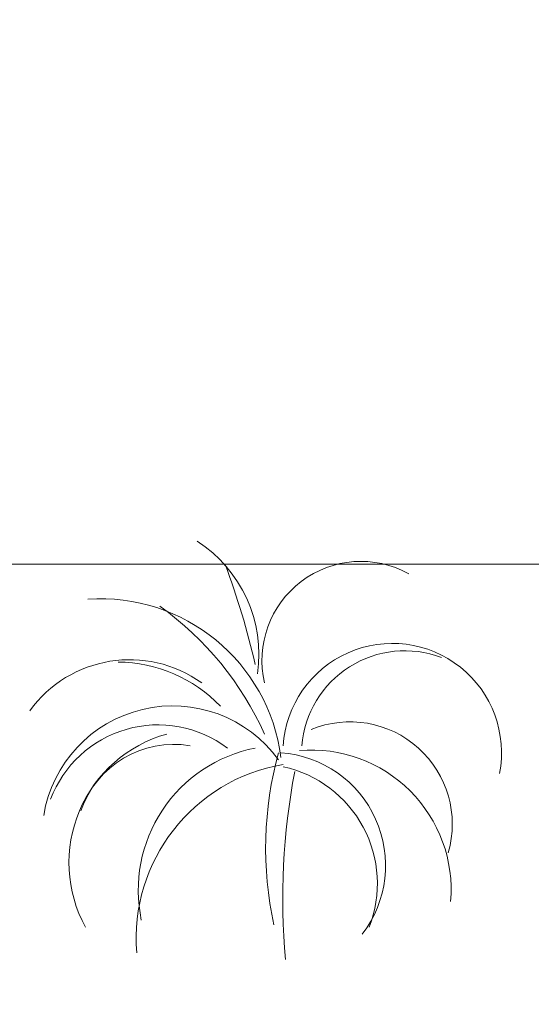
# Model space of a CAD drawing. Units: millimetres. Extents: x 595116 to 630915, y 909473 to 920225.
# Tile 80 of 134: x 629661 to 629703, y 919267 to 919346. Entities that reach past the tile are written whole.
import ezdxf

# ---------------------------------------------------------------- set-up
doc = ezdxf.new("R2010")
doc.units = ezdxf.units.MM
doc.layers.add('Dimension', color=3, linetype='Continuous', lineweight=18)
doc.layers.add('L-PLNT', color=85, linetype='Continuous', lineweight=13)
doc.styles.get("Standard").update_dxf_attribs({"font": 'arial.ttf'})
doc.dimstyles.new('ISO-25', dxfattribs={"dimtxt": 9, "dimasz": 6, "dimexe": 1.25, "dimexo": 0.625, "dimtad": 1, "dimlunit": 4, "dimtxsty": 'Standard', "dimcen": 2.5, "dimadec": 0, "dimazin": 0, "dimtfac": 1, "dimtmove": 0, "dimatfit": 3, "dimfxl": 1, "dimarcsym": 0})

# ---------------------------------------------------------------- blocks, each defined once
blk = doc.blocks.new('tree')
for centre, radius, start, end in [((629595.141, 919296.95), 5.184, 352.032, 57.0714), ((629604.232, 919296.737), 3.791, 61.1347, 193.108), ((629569.835, 919289.496), 31.168, 13.149, 20.5076), ((629594.259, 919292.132), 6.965, 7.4001, 94.0059), ((629589.446, 919288.922), 12.167, 24.2477, 54.3726), ((629605.429, 919293.205), 4.185, 348.9977, 176.315), ((629605.915, 919293.144), 3.963, 69.3845, 175.231), ((629595.377, 919292.044), 4.722, 54.2484, 144.2167), ((629594.88, 919291.171), 5.506, 43.8672, 89.4805), ((629597.025, 919289.989), 5.01, 36.0581, 170.6542), ((629596.464, 919289.874), 4.4, 52.9074, 159.3471), ((629603.809, 919290.469), 3.92, 343.886, 112.2662), ((629598.153, 919288.998), 5.103, 105.3576, 208.8973), ((629597.068, 919289.758), 3.768, 80.4816, 161.0664), ((629601.247, 919287.941), 5.545, 101.0419, 191.8692), ((629602.329, 919287.957), 5.355, 355.2141, 94.8217), ((629614.329, 919289.554), 13.748, 164.5925, 192.323), ((629600.849, 919288.894), 4.324, 322.5461, 85.805), ((629602.391, 919286.088), 6.769, 99.681, 184.5451), ((629600.275, 919288.191), 4.585, 338.7925, 77.6921), ((629626.813, 919287.645), 25.579, 169.0753, 185.2889)]:
    blk.add_arc(centre, radius, start, end)
blk = doc.blocks.new('*D216')
at = {"layer": 'Defpoints', "color": 0, "transparency": 16777216}
for p in [(629505.041, 919411.828), (629743.541, 919411.928), (629743.541, 918832.378)]:
    blk.add_point(p, dxfattribs=at)
at = {"layer": 'Dimension', "color": 0, "lineweight": -2, "transparency": 16777216}
for p, q in [((629505.041, 919411.203), (629505.041, 918831.128)), ((629743.541, 919411.303), (629743.541, 918831.128)), ((629511.041, 918832.378), (629737.541, 918832.378))]:
    blk.add_line(p, q, dxfattribs=at)
at = {"layer": 'Dimension', "color": 0, "transparency": 16777216}
for points in [[(629511.041, 918833.378), (629511.041, 918831.378), (629505.041, 918832.378)], [(629737.541, 918833.378), (629737.541, 918831.378), (629743.541, 918832.378)]]:
    blk.add_solid(points, dxfattribs=at)
at = {"layer": 'Dimension', "color": 0, "transparency": 16777216, "insert": (629624.291, 918837.656), "char_height": 9, "attachment_point": 5}
blk.add_mtext('19\'-10 1/2"', dxfattribs=at)
blk = doc.blocks.new('*D220')
at = {"layer": 'Defpoints', "color": 0, "transparency": 16777216}
for p in [(629824.951, 920160.756), (629511.274, 919302.009), (629824.951, 919302.009)]:
    blk.add_point(p, dxfattribs=at)
at = {"layer": 'Dimension', "color": 0, "lineweight": -2, "transparency": 16777216}
for p, q in [((629511.274, 919302.634), (629511.274, 920162.006)), ((629824.951, 919302.634), (629824.951, 920162.006)), ((629517.274, 920160.756), (629818.951, 920160.756))]:
    blk.add_line(p, q, dxfattribs=at)
at = {"layer": 'Dimension', "color": 0, "transparency": 16777216}
for points in [[(629517.274, 920161.756), (629517.274, 920159.756), (629511.274, 920160.756)], [(629818.951, 920161.756), (629818.951, 920159.756), (629824.951, 920160.756)]]:
    blk.add_solid(points, dxfattribs=at)
at = {"layer": 'Dimension', "color": 0, "transparency": 16777216, "insert": (629668.113, 920166.035), "char_height": 9, "attachment_point": 5}
blk.add_mtext('26\'-1 1/2"', dxfattribs=at)

msp = doc.modelspace()

# ---------------------------------------------------------------- linework, layer by layer
at = {"layer": 'L-PLNT'}
msp.add_line((629824.951, 919302.009), (629511.274, 919302.009), dxfattribs=at)

# ---------------------------------------------------------------- block references
at = {"layer": 'L-PLNT', "xscale": 2.107689410566463, "yscale": 2.107689410566463, "zscale": 2.107689410566463}
msp.add_blockref('tree', (-697321.173, -1018297.752), dxfattribs=at)

# ---------------------------------------------------------------- dimensions: what is measured, and where the dimension line sits
at = {"layer": 'Dimension'}
for base, p1, p2, picture, middle in [((629824.951, 920160.756), (629511.274, 919302.009), (629824.951, 919302.009), '*D220', (629668.113, 920166.035)), ((629743.541, 918832.378), (629505.041, 919411.828), (629743.541, 919411.928), '*D216', (629624.291, 918837.656))]:
    dim = msp.add_linear_dim(base=base, p1=p1, p2=p2, dimstyle='ISO-25', override={"dimdec": 1, "dimlfac": 1, "dimrnd": 0, "dimzin": 1, "dimdsep": 46, "dimlunit": 4, "dimfrac": 2}, dxfattribs=at)
    dim.commit()
    dim.dimension.update_dxf_attribs({"geometry": picture, "text_midpoint": middle})

doc.saveas('drawing.dxf')
